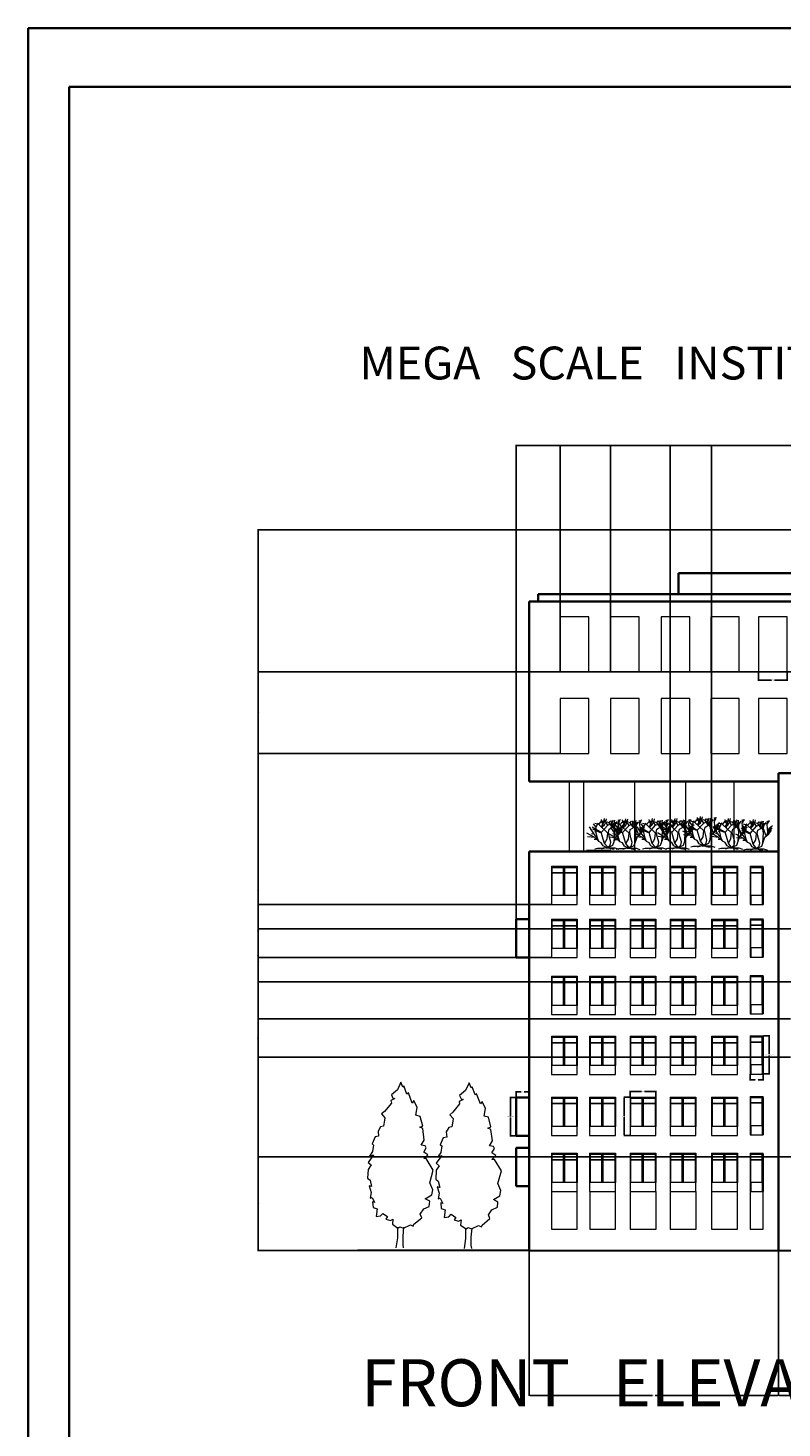
# Model space of a CAD drawing. Units: inches. Extents: x -279 to 364, y -385 to 335.
# Tile 5 of 9: x -279 to -60, y -72 to 335. Entities that reach past the tile are written whole.
import ezdxf

# ---------------------------------------------------------------- set-up
doc = ezdxf.new("R2010")
doc.units = ezdxf.units.IN
doc.header["$MEASUREMENT"] = 0
for name, color, linetype, lineweight in [('A-ANNO-DIMS', 2, 'Continuous', 18), ('A-ANNO-TEXT', 7, 'Continuous', 25), ('A-ANNO-TTLB', 7, 'Continuous', 35), ('A-GLAZ', 4, 'Continuous', 18), ('A-GLAZ-CURT', 4, 'Continuous', 18), ('A-ROOF', 7, 'Continuous', 35), ('A-WALL', 7, 'Continuous', 35), ('C-TOPO', 32, 'Continuous', 30), ('L-PLNT', 94, 'Continuous', 13)]:
    doc.layers.add(name, color=color, linetype=linetype, lineweight=lineweight)
doc.styles.get("Standard").update_dxf_attribs({"font": 'arial.ttf'})
doc.dimstyles.get("Standard").update_dxf_attribs({"dimtxt": 0.18, "dimasz": 0.18, "dimexe": 0.18, "dimexo": 0.0625, "dimgap": 0.09, "dimtad": 0, "dimtih": 1, "dimtoh": 1, "dimdec": 4, "dimzin": 0, "dimdsep": 46, "dimtxsty": 'Standard', "dimcen": 0.09, "dimadec": 0, "dimazin": 0, "dimtfac": 1, "dimtdec": 4, "dimtofl": 0, "dimtmove": 0, "dimatfit": 3, "dimfxl": 1, "dimtolj": 1, "dimtzin": 0, "dimarcsym": 0})

# ---------------------------------------------------------------- blocks, each defined once
blk = doc.blocks.new('*U2')
for p, q in [((-12.471, 19.775), (-12.898, 22.044)), ((-11.28, 19.619), (-12.104, 21.184)), ((-11.433, 18.289), (-10.457, 22.749)), ((-8.16, 17.76), (-10.56, 21.6)), ((-9.48, 19.775), (-8.992, 22.592)), ((-7.2, 19.68), (-6.24, 21.12)), ((-5.086, 17.741), (-5.513, 21.34)), ((-5.28, 19.2), (-3.84, 21.6)), ((-3.377, 18.602), (-2.888, 21.575)), ((-0.508, 21.888), (-0.081, 20.558)), ((-0.203, 19.149), (0.102, 21.34)), ((-0.02, 20.01), (0.896, 21.105)), ((0.041, 20.714), (1.384, 22.044)), ((0.102, 21.34), (0.835, 21.888)), ((-17.76, 8.64), (-23.663, 11.961)), ((-18.24, 11.04), (-21.755, 16.655)), ((-18.24, 11.04), (-20.16, 11.52)), ((-12.96, 12.48), (-19.68, 16.32)), ((-13.92, 12.48), (-19.2, 14.88)), ((-16.8, 16.32), (-18.72, 18.72)), ((-15.84, 8.16), (-18.24, 11.04)), ((-14.88, 18.24), (-17.76, 19.2)), ((-16.8, 12.48), (-17.76, 12.96)), ((-16.8, 16.32), (-15.36, 19.68)), ((-16.8, 12.48), (-16.8, 16.32)), ((-15.84, 8.16), (-16.8, 12.48)), ((-14.88, 18.24), (-12.96, 20.64)), ((-8.16, 12), (-14.88, 18.24)), ((-12.96, 12.48), (-13.92, 12.48)), ((-13.325, 16.724), (-11.433, 18.289)), ((-12.96, 12.48), (-8.16, 17.76)), ((-10.56, 4.32), (-12.96, 12.48)), ((-11.677, 19.071), (-12.471, 19.775)), ((-12.043, 15.628), (-11.921, 18.836)), ((-11.982, 16.802), (-10.579, 18.054)), ((-11.921, 18.836), (-10.64, 20.401)), ((-10.579, 18.054), (-9.846, 19.697)), ((-7.2, 19.68), (-8.64, 20.16)), ((-8.64, 7.68), (-8.16, 12)), ((-8.16, 17.76), (-5.28, 19.2)), ((-7.68, 12.48), (-7.2, 14.88)), ((-6.72, 8.64), (-7.68, 12.48)), ((-4.8, 16.32), (-7.2, 19.68)), ((-7.2, 14.88), (-3.84, 16.8)), ((-3.377, 15.315), (-5.086, 17.819)), ((-2.88, 12.96), (-4.32, 19.68)), ((-3.84, 16.8), (-0.96, 20.64)), ((-2.766, 16.802), (-3.377, 18.602)), ((-3.36, 5.28), (-2.88, 12.96)), ((-2.88, 15.84), (-2.4, 20.16)), ((-0.96, 10.56), (-2.88, 15.84)), ((-1.92, 9.6), (0.96, 12)), ((-0.48, 10.8), (0.346, 13.203)), ((0.346, 13.203), (-0.203, 19.149)), ((-0.142, 19.384), (0.59, 20.401)), ((0.346, 13.203), (1.323, 16.254)), ((0.96, 12), (1.44, 15.36)), ((0.96, 12), (2.88, 14.88)), ((1.323, 16.254), (3.642, 18.289)), ((1.44, 15.36), (2.88, 17.28)), ((1.92, 13.44), (2.4, 15.36)), ((2.4, 15.36), (3.36, 16.32)), ((-17.76, 8.64), (-23.128, 9.222)), ((-16.32, 7.2), (-18.24, 7.2)), ((-14.88, 5.76), (-17.76, 8.64)), ((-15.84, 0.48), (-17.76, 0)), ((-14.88, 5.76), (-15.84, 8.16)), ((-13.44, 0.48), (-15.84, 0.48)), ((-12.96, 4.8), (-14.88, 5.76)), ((-9.6, 0.96), (-13.44, 0.48)), ((-11.52, 2.4), (-12.96, 4.8)), ((-9.6, 0.96), (-12.96, 0)), ((-8.64, 0.96), (-11.52, 2.4)), ((-10.56, 4.32), (-8.64, 7.68)), ((-8.64, 1.92), (-10.56, 4.32)), ((-9.6, 0.96), (-7.68, 0.96)), ((-8.64, 0.96), (-4.32, 2.88)), ((-8.64, 0.96), (-6.24, 2.88)), ((-8.64, 0.96), (-8.64, 1.92)), ((-8.64, 0.96), (-2.88, 0.96)), ((-7.68, 0.96), (-6.24, 0.48)), ((-5.76, 5.28), (-6.72, 8.64)), ((-6.24, 2.88), (-5.76, 5.28)), ((-6.24, 0.48), (-3.36, 0)), ((-4.32, 2.88), (-1.92, 9.6)), ((-2.88, 0.96), (0, 0))]:
    blk.add_line(p, q)
blk = doc.blocks.new('*U3')
blk.add_lwpolyline([(-2.754, 191.699), (-6.78, 182.851), (-13.682, 176.953), (-11.956, 173.266), (-9.656, 172.529), (-14.257, 170.317), (-13.682, 167.368), (-21.733, 157.783), (-25.184, 154.834), (-21.158, 150.41), (-21.733, 147.461), (-22.884, 140.825), (-26.334, 140.087), (-29.21, 134.926), (-28.635, 129.028), (-32.661, 128.291), (-36.111, 120.18), (-34.386, 118.706), (-35.536, 111.333), (-38.987, 106.171), (-34.386, 107.646), (-40.712, 98.798), (-37.261, 95.849), (-40.712, 90.688), (-41.287, 80.366), (-38.412, 78.154), (-36.686, 70.781), (-39.562, 71.518), (-37.261, 64.145), (-38.412, 57.509), (-36.111, 58.247), (-33.236, 52.348), (-35.536, 53.086), (-34.961, 46.45), (-30.36, 44.975), (-31.51, 36.128), (-26.334, 36.865), (-23.459, 39.814), (-18.283, 36.128), (-20.008, 33.178), (-14.832, 31.704), (-11.956, 33.178), (-12.531, 27.28), (-6.205, 22.856), (-3.905, 24.331), (0.121, 22.856), (8.173, 26.543), (11.624, 25.068), (12.199, 27.28), (21.4, 34.653), (19.675, 39.077), (23.701, 44.975), (30.027, 47.924), (30.602, 53.823), (25.426, 56.772), (32.903, 61.196), (34.053, 67.094), (30.602, 75.205), (34.628, 89.951), (26.576, 103.222), (23.701, 103.222), (28.302, 107.646), (23.701, 110.595), (26.576, 115.756), (25.426, 117.968), (20.825, 118.706), (24.276, 124.604), (22.551, 137.876), (19.1, 139.35), (22.551, 140.825), (19.675, 151.884), (14.499, 153.359), (16.224, 162.207), (12.199, 170.317), (10.473, 167.368), (5.872, 179.165), (4.147, 177.69), (0.696, 187.275), (-0.454, 185.8)], close=True)
for points in [[(-6.813, 23.669), (-6.813, 11.669), (-8.627, 0)], [(0.387, 23.669), (-0.576, 13.271), (-0.576, 3.686), (0, 0)]]:
    blk.add_lwpolyline(points)
blk = doc.blocks.new('WIN-WING-NARROW')
for p, q in [((0, 11.12), (0, 0)), ((0, 11.12), (3.85, 11.12)), ((0.2, 2.62), (0.2, 10.81)), ((0.2, 10.81), (3.85, 10.81)), ((0.2, 9.34), (3.52, 9.34)), ((0.2, 9.24), (3.52, 9.24)), ((3.52, 9.34), (3.52, 10.81)), ((3.52, 2.62), (3.52, 9.24)), ((3.85, 9.24), (3.85, 11.12)), ((3.85, 10.81), (3.85, 9.34)), ((3.85, 9.24), (3.85, 2.62)), ((3.85, 2.62), (0, 2.62)), ((0, 0), (3.85, 0)), ((0.2, 2.62), (0.2, 0)), ((3.52, 2.62), (3.52, 0)), ((3.85, 2.62), (3.85, 0))]:
    blk.add_line(p, q)
blk = doc.blocks.new('WIN-TOWER-FRONT')
for p, q in [((8.3, 15.93), (0, 15.93)), ((0, 15.93), (0, 14.74)), ((0, 14.74), (0, 0)), ((8.3, 0), (8.3, 15.93)), ((0, 0), (8.3, 0))]:
    blk.add_line(p, q)
blk = doc.blocks.new('WING-RETURN-SHORT')
for p, q in [((3.76, 11.12), (0, 11.12)), ((0, 11.12), (0, 0)), ((0, 0), (3.76, 0))]:
    blk.add_line(p, q)
blk = doc.blocks.new('WIN-WING-TWIN')
for p, q in [((0, 11.12), (0, 0)), ((0, 11.12), (7.53, 11.12)), ((0.2, 2.62), (0.2, 10.81)), ((0.2, 10.81), (7.32, 10.81)), ((0.2, 9.34), (3.52, 9.34)), ((0.2, 9.24), (3.52, 9.24)), ((3.52, 9.34), (3.52, 10.81)), ((3.52, 2.62), (3.52, 9.24)), ((3.85, 10.81), (3.85, 9.34)), ((3.85, 9.34), (7.32, 9.34)), ((3.85, 9.24), (7.32, 9.24)), ((3.85, 9.24), (3.85, 2.62)), ((7.32, 10.81), (7.32, 2.62)), ((7.53, 11.12), (7.53, 2.62)), ((7.53, 2.62), (0, 2.62)), ((0, 0), (7.53, 0)), ((7.53, 0), (7.53, 2.62))]:
    blk.add_line(p, q)
blk = doc.blocks.new('*D30')
at = {"layer": 'A-ANNO-DIMS', "color": 0, "lineweight": -2, "transparency": 16777216}
for p, q in [((-104.61, 24.4), (-106.39, 24.4)), ((-106.21, 24.22), (-106.21, 19.02)), ((-106.21, 13.46), (-106.21, 18.66)), ((-104.61, 13.28), (-106.39, 13.28))]:
    blk.add_line(p, q, dxfattribs=at)
at = {"layer": 'A-ANNO-DIMS', "color": 0, "transparency": 16777216}
for points in [[(-106.24, 24.22), (-106.18, 24.22), (-106.21, 24.4)], [(-106.24, 13.46), (-106.18, 13.46), (-106.21, 13.28)]]:
    blk.add_solid(points, dxfattribs=at)
at = {"layer": 'Defpoints', "color": 0, "transparency": 16777216}
for p in [(-106.21, 24.4), (-104.55, 24.4), (-104.55, 13.28)]:
    blk.add_point(p, dxfattribs=at)
at = {"layer": 'A-ANNO-DIMS', "color": 0, "transparency": 16777216, "insert": (-106.21, 18.84), "char_height": 0.18, "attachment_point": 5}
blk.add_mtext('\\A1;PAIR 11 TYP.', dxfattribs=at)
blk = doc.blocks.new('*D31')
at = {"layer": 'A-ANNO-DIMS', "color": 0, "lineweight": -2, "transparency": 16777216}
for p, q in [((-104.55, 24.46), (-104.55, 26.25)), ((-104.37, 26.07), (-101.24, 26.07)), ((-97.2, 26.07), (-100.32, 26.07)), ((-97.02, 24.46), (-97.02, 26.25))]:
    blk.add_line(p, q, dxfattribs=at)
at = {"layer": 'A-ANNO-DIMS', "color": 0, "transparency": 16777216}
for points in [[(-104.37, 26.1), (-104.37, 26.04), (-104.55, 26.07)], [(-97.2, 26.1), (-97.2, 26.04), (-97.02, 26.07)]]:
    blk.add_solid(points, dxfattribs=at)
at = {"layer": 'Defpoints', "color": 0, "transparency": 16777216}
for p in [(-104.55, 24.4), (-97.02, 26.07), (-97.02, 24.4)]:
    blk.add_point(p, dxfattribs=at)
at = {"layer": 'A-ANNO-DIMS', "color": 0, "transparency": 16777216, "insert": (-100.78, 26.07), "char_height": 0.18, "attachment_point": 5}
blk.add_mtext('\\A1;8 TYP.', dxfattribs=at)
blk = doc.blocks.new('*D32')
at = {"layer": 'A-ANNO-DIMS', "color": 0, "lineweight": -2, "transparency": 16777216}
for p, q in [((-65.82, 42.24), (-64.03, 42.24)), ((-64.21, 42.06), (-64.21, 36.87)), ((-64.21, 31.31), (-64.21, 36.5)), ((-65.82, 31.13), (-64.03, 31.13))]:
    blk.add_line(p, q, dxfattribs=at)
at = {"layer": 'A-ANNO-DIMS', "color": 0, "transparency": 16777216}
for points in [[(-64.24, 42.06), (-64.18, 42.06), (-64.21, 42.24)], [(-64.24, 31.31), (-64.18, 31.31), (-64.21, 31.13)]]:
    blk.add_solid(points, dxfattribs=at)
at = {"layer": 'Defpoints', "color": 0, "transparency": 16777216}
for p in [(-65.88, 42.24), (-64.21, 42.24), (-65.88, 31.13)]:
    blk.add_point(p, dxfattribs=at)
at = {"layer": 'A-ANNO-DIMS', "color": 0, "transparency": 16777216, "insert": (-64.21, 36.68), "char_height": 0.18, "attachment_point": 5}
blk.add_mtext('\\A1;NARROW SASH 11 TYP.', dxfattribs=at)
blk = doc.blocks.new('*D33')
at = {"layer": 'A-ANNO-DIMS', "color": 0, "lineweight": -2, "transparency": 16777216}
for p, q in [((-69.73, 31.06), (-69.73, 29.28)), ((-69.55, 29.46), (-68.26, 29.46)), ((-66.06, 29.46), (-67.34, 29.46)), ((-65.88, 31.06), (-65.88, 29.28))]:
    blk.add_line(p, q, dxfattribs=at)
at = {"layer": 'A-ANNO-DIMS', "color": 0, "transparency": 16777216}
for points in [[(-69.55, 29.49), (-69.55, 29.43), (-69.73, 29.46)], [(-66.06, 29.49), (-66.06, 29.43), (-65.88, 29.46)]]:
    blk.add_solid(points, dxfattribs=at)
at = {"layer": 'Defpoints', "color": 0, "transparency": 16777216}
for p in [(-69.73, 31.13), (-65.88, 31.13), (-65.88, 29.46)]:
    blk.add_point(p, dxfattribs=at)
at = {"layer": 'A-ANNO-DIMS', "color": 0, "transparency": 16777216, "insert": (-67.8, 29.46), "char_height": 0.18, "attachment_point": 5}
blk.add_mtext('\\A1;4 TYP.', dxfattribs=at)
blk = doc.blocks.new('*D35')
at = {"layer": 'A-ANNO-DIMS', "color": 0, "lineweight": -2, "transparency": 16777216}
for p, q in [((-67.23, 147.75), (-67.23, 145.25)), ((-58.93, 147.75), (-58.93, 145.25)), ((-67.05, 145.43), (-63.54, 145.43)), ((-59.11, 145.43), (-62.62, 145.43))]:
    blk.add_line(p, q, dxfattribs=at)
at = {"layer": 'A-ANNO-DIMS', "color": 0, "transparency": 16777216}
for points in [[(-67.05, 145.46), (-67.05, 145.4), (-67.23, 145.43)], [(-59.11, 145.46), (-59.11, 145.4), (-58.93, 145.43)]]:
    blk.add_solid(points, dxfattribs=at)
at = {"layer": 'Defpoints', "color": 0, "transparency": 16777216}
for p in [(-67.23, 147.82), (-58.93, 147.82), (-58.93, 145.43)]:
    blk.add_point(p, dxfattribs=at)
at = {"layer": 'A-ANNO-DIMS', "color": 0, "transparency": 16777216, "insert": (-63.08, 145.43), "char_height": 0.18, "attachment_point": 5}
blk.add_mtext('\\A1;8 TYP.', dxfattribs=at)
blk = doc.blocks.new('*D64')
at = {"layer": 'A-ANNO-DIMS', "color": 0, "lineweight": -2, "transparency": 16777216}
for p, q in [((-137.62, 24.27), (-139.41, 24.27)), ((-139.23, 24.09), (-139.23, 18.9)), ((-139.23, 13.34), (-139.23, 18.53)), ((-137.62, 13.16), (-139.41, 13.16))]:
    blk.add_line(p, q, dxfattribs=at)
at = {"layer": 'A-ANNO-DIMS', "color": 0, "transparency": 16777216}
for points in [[(-139.26, 24.09), (-139.2, 24.09), (-139.23, 24.27)], [(-139.26, 13.34), (-139.2, 13.34), (-139.23, 13.16)]]:
    blk.add_solid(points, dxfattribs=at)
at = {"layer": 'Defpoints', "color": 0, "transparency": 16777216}
for p in [(-139.23, 24.27), (-137.56, 24.27), (-137.56, 13.16)]:
    blk.add_point(p, dxfattribs=at)
at = {"layer": 'A-ANNO-DIMS', "color": 0, "transparency": 16777216, "insert": (-139.23, 18.71), "char_height": 0.18, "attachment_point": 5}
blk.add_mtext('\\A1;RETURN 11 TYP.', dxfattribs=at)
blk = doc.blocks.new('*D65')
at = {"layer": 'A-ANNO-DIMS', "color": 0, "lineweight": -2, "transparency": 16777216}
for p, q in [((-137.56, 24.33), (-137.56, 26.12)), ((-137.38, 25.94), (-136.14, 25.94)), ((-133.98, 25.94), (-135.22, 25.94)), ((-133.8, 24.33), (-133.8, 26.12))]:
    blk.add_line(p, q, dxfattribs=at)
at = {"layer": 'A-ANNO-DIMS', "color": 0, "transparency": 16777216}
for points in [[(-137.38, 25.97), (-137.38, 25.91), (-137.56, 25.94)], [(-133.98, 25.97), (-133.98, 25.91), (-133.8, 25.94)]]:
    blk.add_solid(points, dxfattribs=at)
at = {"layer": 'Defpoints', "color": 0, "transparency": 16777216}
for p in [(-133.8, 25.94), (-137.56, 24.27), (-133.8, 24.27)]:
    blk.add_point(p, dxfattribs=at)
at = {"layer": 'A-ANNO-DIMS', "color": 0, "transparency": 16777216, "insert": (-135.68, 25.94), "char_height": 0.18, "attachment_point": 5}
blk.add_mtext('\\A1;4 TYP.', dxfattribs=at)
blk = doc.blocks.new('*D74')
at = {"layer": 'A-ANNO-DIMS', "color": 0, "lineweight": -2, "transparency": 16777216}
for p, q in [((-137.56, 76.08), (-137.56, 213.67)), ((-137.38, 213.49), (54.29, 213.49)), ((246.75, 213.49), (55.08, 213.49)), ((246.93, 76.27), (246.93, 213.67))]:
    blk.add_line(p, q, dxfattribs=at)
at = {"layer": 'A-ANNO-DIMS', "color": 0, "transparency": 16777216}
for points in [[(-137.38, 213.52), (-137.38, 213.46), (-137.56, 213.49)], [(246.75, 213.52), (246.75, 213.46), (246.93, 213.49)]]:
    blk.add_solid(points, dxfattribs=at)
at = {"layer": 'Defpoints', "color": 0, "transparency": 16777216}
for p in [(246.93, 213.49), (-137.56, 76.01), (246.93, 76.21)]:
    blk.add_point(p, dxfattribs=at)
at = {"layer": 'A-ANNO-DIMS', "color": 0, "transparency": 16777216, "insert": (54.68, 213.49), "char_height": 0.18, "attachment_point": 5}
blk.add_mtext('\\A1;384.5', dxfattribs=at)
blk = doc.blocks.new('*D75')
at = {"layer": 'A-ANNO-DIMS', "color": 0, "lineweight": -2, "transparency": 16777216}
for p, q in [((53.76, 188.99), (-212.62, 188.99)), ((-212.44, 188.81), (-212.44, 84.64)), ((-212.44, -19.9), (-212.44, 84.27)), ((-133.86, -20.08), (-212.62, -20.08))]:
    blk.add_line(p, q, dxfattribs=at)
at = {"layer": 'A-ANNO-DIMS', "color": 0, "transparency": 16777216}
for points in [[(-212.47, 188.81), (-212.41, 188.81), (-212.44, 188.99)], [(-212.47, -19.9), (-212.41, -19.9), (-212.44, -20.08)]]:
    blk.add_solid(points, dxfattribs=at)
at = {"layer": 'Defpoints', "color": 0, "transparency": 16777216}
for p in [(-212.44, 188.99), (53.82, 188.99), (-133.8, -20.08)]:
    blk.add_point(p, dxfattribs=at)
at = {"layer": 'A-ANNO-DIMS', "color": 0, "transparency": 16777216, "insert": (-212.44, 84.45), "char_height": 0.18, "attachment_point": 5}
blk.add_mtext('\\A1;209.07', dxfattribs=at)
blk = doc.blocks.new('*D76')
at = {"layer": 'A-ANNO-DIMS', "color": 0, "lineweight": -2, "transparency": 16777216}
for p, q in [((17.12, 147.82), (-212.62, 147.82)), ((-212.44, 147.64), (-212.44, 64.05)), ((-212.44, -19.9), (-212.44, 63.68)), ((17.4, -20.08), (-212.62, -20.08))]:
    blk.add_line(p, q, dxfattribs=at)
at = {"layer": 'A-ANNO-DIMS', "color": 0, "transparency": 16777216}
for points in [[(-212.47, 147.64), (-212.41, 147.64), (-212.44, 147.82)], [(-212.47, -19.9), (-212.41, -19.9), (-212.44, -20.08)]]:
    blk.add_solid(points, dxfattribs=at)
at = {"layer": 'Defpoints', "color": 0, "transparency": 16777216}
for p in [(-212.44, 147.82), (17.19, 147.82), (17.46, -20.08)]:
    blk.add_point(p, dxfattribs=at)
at = {"layer": 'A-ANNO-DIMS', "color": 0, "transparency": 16777216, "insert": (-212.44, 63.87), "char_height": 0.18, "attachment_point": 5}
blk.add_mtext('\\A1;167.9', dxfattribs=at)
blk = doc.blocks.new('*D77')
at = {"layer": 'A-ANNO-DIMS', "color": 0, "lineweight": -2, "transparency": 16777216}
for p, q in [((-133.8, -20.14), (-133.8, -62.3)), ((-61.49, -20.14), (-61.49, -62.3)), ((-133.62, -62.12), (-98.02, -62.12)), ((-61.67, -62.12), (-97.27, -62.12))]:
    blk.add_line(p, q, dxfattribs=at)
at = {"layer": 'A-ANNO-DIMS', "color": 0, "transparency": 16777216}
for points in [[(-133.62, -62.09), (-133.62, -62.15), (-133.8, -62.12)], [(-61.67, -62.09), (-61.67, -62.15), (-61.49, -62.12)]]:
    blk.add_solid(points, dxfattribs=at)
at = {"layer": 'Defpoints', "color": 0, "transparency": 16777216}
for p in [(-133.8, -20.08), (-61.49, -20.08), (-61.49, -62.12)]:
    blk.add_point(p, dxfattribs=at)
at = {"layer": 'A-ANNO-DIMS', "color": 0, "transparency": 16777216, "insert": (-97.64, -62.12), "char_height": 0.18, "attachment_point": 5}
blk.add_mtext('\\A1;72.31', dxfattribs=at)
blk = doc.blocks.new('*D78')
at = {"layer": 'A-ANNO-DIMS', "color": 0, "lineweight": -2, "transparency": 16777216}
for p, q in [((-61.49, -20.14), (-61.49, -62.3)), ((13.58, -20.14), (13.58, -62.3)), ((-61.31, -62.12), (-24.34, -62.12)), ((13.4, -62.12), (-23.56, -62.12))]:
    blk.add_line(p, q, dxfattribs=at)
at = {"layer": 'A-ANNO-DIMS', "color": 0, "transparency": 16777216}
for points in [[(-61.31, -62.09), (-61.31, -62.15), (-61.49, -62.12)], [(13.4, -62.09), (13.4, -62.15), (13.58, -62.12)]]:
    blk.add_solid(points, dxfattribs=at)
at = {"layer": 'Defpoints', "color": 0, "transparency": 16777216}
for p in [(-61.49, -20.08), (13.58, -20.08), (13.58, -62.12)]:
    blk.add_point(p, dxfattribs=at)
at = {"layer": 'A-ANNO-DIMS', "color": 0, "transparency": 16777216, "insert": (-23.95, -62.12), "char_height": 0.18, "attachment_point": 5}
blk.add_mtext('\\A1;75.07', dxfattribs=at)
blk = doc.blocks.new('*D85')
at = {"layer": 'A-ANNO-DIMS', "color": 0, "lineweight": -2, "transparency": 16777216}
for p, q in [((-124.8, 147.88), (-124.8, 213.67)), ((-124.62, 213.49), (-117.91, 213.49)), ((-110.43, 213.49), (-117.14, 213.49)), ((-110.25, 147.88), (-110.25, 213.67))]:
    blk.add_line(p, q, dxfattribs=at)
at = {"layer": 'A-ANNO-DIMS', "color": 0, "transparency": 16777216}
for points in [[(-124.62, 213.52), (-124.62, 213.46), (-124.8, 213.49)], [(-110.43, 213.52), (-110.43, 213.46), (-110.25, 213.49)]]:
    blk.add_solid(points, dxfattribs=at)
at = {"layer": 'Defpoints', "color": 0, "transparency": 16777216}
for p in [(-110.25, 213.49), (-124.8, 147.82), (-110.25, 147.82)]:
    blk.add_point(p, dxfattribs=at)
at = {"layer": 'A-ANNO-DIMS', "color": 0, "transparency": 16777216, "insert": (-117.52, 213.49), "char_height": 0.18, "attachment_point": 5}
blk.add_mtext('\\A1;14.55', dxfattribs=at)
blk = doc.blocks.new('*D86')
at = {"layer": 'A-ANNO-DIMS', "color": 0, "lineweight": -2, "transparency": 16777216}
for p, q in [((-124.86, 147.82), (-212.62, 147.82)), ((-212.44, 147.64), (-212.44, 136.17)), ((-212.44, 124.35), (-212.44, 135.81)), ((-124.86, 124.17), (-212.62, 124.17))]:
    blk.add_line(p, q, dxfattribs=at)
at = {"layer": 'A-ANNO-DIMS', "color": 0, "transparency": 16777216}
for points in [[(-212.47, 147.64), (-212.41, 147.64), (-212.44, 147.82)], [(-212.47, 124.35), (-212.41, 124.35), (-212.44, 124.17)]]:
    blk.add_solid(points, dxfattribs=at)
at = {"layer": 'Defpoints', "color": 0, "transparency": 16777216}
for p in [(-212.44, 147.82), (-124.8, 147.82), (-124.8, 124.17)]:
    blk.add_point(p, dxfattribs=at)
at = {"layer": 'A-ANNO-DIMS', "color": 0, "transparency": 16777216, "insert": (-212.44, 135.99), "char_height": 0.18, "attachment_point": 5}
blk.add_mtext('\\A1;23.646', dxfattribs=at)
blk = doc.blocks.new('*D87')
at = {"layer": 'A-ANNO-DIMS', "color": 0, "lineweight": -2, "transparency": 16777216}
for p, q in [((-92.95, 80.34), (-92.95, 213.67)), ((-92.77, 213.49), (-87.37, 213.49)), ((-81.05, 213.49), (-86.46, 213.49)), ((-80.87, 80.34), (-80.87, 213.67))]:
    blk.add_line(p, q, dxfattribs=at)
at = {"layer": 'A-ANNO-DIMS', "color": 0, "transparency": 16777216}
for points in [[(-92.77, 213.52), (-92.77, 213.46), (-92.95, 213.49)], [(-81.05, 213.52), (-81.05, 213.46), (-80.87, 213.49)]]:
    blk.add_solid(points, dxfattribs=at)
at = {"layer": 'Defpoints', "color": 0, "transparency": 16777216}
for p in [(-80.87, 213.49), (-92.95, 80.27), (-80.87, 80.27)]:
    blk.add_point(p, dxfattribs=at)
at = {"layer": 'A-ANNO-DIMS', "color": 0, "transparency": 16777216, "insert": (-86.91, 213.49), "char_height": 0.18, "attachment_point": 5}
blk.add_mtext('\\A1;12.082', dxfattribs=at)
blk = doc.blocks.new('*D88')
at = {"layer": 'A-ANNO-DIMS', "color": 0, "lineweight": -2, "transparency": 16777216}
for p, q in [((-127.43, 80.27), (-212.62, 80.27)), ((-212.44, 80.09), (-212.44, 72.77)), ((-212.44, 65.08), (-212.44, 72.4)), ((-127.43, 64.9), (-212.62, 64.9))]:
    blk.add_line(p, q, dxfattribs=at)
at = {"layer": 'A-ANNO-DIMS', "color": 0, "transparency": 16777216}
for points in [[(-212.47, 80.09), (-212.41, 80.09), (-212.44, 80.27)], [(-212.47, 65.08), (-212.41, 65.08), (-212.44, 64.9)]]:
    blk.add_solid(points, dxfattribs=at)
at = {"layer": 'Defpoints', "color": 0, "transparency": 16777216}
for p in [(-127.37, 80.27), (-212.44, 64.9), (-127.37, 64.9)]:
    blk.add_point(p, dxfattribs=at)
at = {"layer": 'A-ANNO-DIMS', "color": 0, "transparency": 16777216, "insert": (-212.44, 72.59), "char_height": 0.18, "attachment_point": 5}
blk.add_mtext('\\A1;15.377', dxfattribs=at)
blk = doc.blocks.new('*D90')
at = {"layer": 'A-ANNO-DIMS', "color": 0, "lineweight": -2, "transparency": 16777216}
for p, q in [((-58.02, 47.17), (-212.62, 47.17)), ((-212.44, 46.99), (-212.44, 41.78)), ((-212.44, 36.2), (-212.44, 41.41)), ((-58.02, 36.02), (-212.62, 36.02))]:
    blk.add_line(p, q, dxfattribs=at)
at = {"layer": 'A-ANNO-DIMS', "color": 0, "transparency": 16777216}
for points in [[(-212.47, 46.99), (-212.41, 46.99), (-212.44, 47.17)], [(-212.47, 36.2), (-212.41, 36.2), (-212.44, 36.02)]]:
    blk.add_solid(points, dxfattribs=at)
at = {"layer": 'Defpoints', "color": 0, "transparency": 16777216}
for p in [(-57.96, 47.17), (-212.44, 36.02), (-57.96, 36.02)]:
    blk.add_point(p, dxfattribs=at)
at = {"layer": 'A-ANNO-DIMS', "color": 0, "transparency": 16777216, "insert": (-212.44, 41.59), "char_height": 0.18, "attachment_point": 5}
blk.add_mtext('\\A1;11.149', dxfattribs=at)
blk = doc.blocks.new('*D91')
at = {"layer": 'A-ANNO-DIMS', "color": 0, "lineweight": -2, "transparency": 16777216}
for p, q in [((-48.59, 73.23), (-212.62, 73.23)), ((-212.44, 73.05), (-212.44, 65.74)), ((-212.44, 58.07), (-212.44, 65.38)), ((-48.59, 57.89), (-212.62, 57.89))]:
    blk.add_line(p, q, dxfattribs=at)
at = {"layer": 'A-ANNO-DIMS', "color": 0, "transparency": 16777216}
for points in [[(-212.47, 73.05), (-212.41, 73.05), (-212.44, 73.23)], [(-212.47, 58.07), (-212.41, 58.07), (-212.44, 57.89)]]:
    blk.add_solid(points, dxfattribs=at)
at = {"layer": 'Defpoints', "color": 0, "transparency": 16777216}
for p in [(-212.44, 73.23), (-48.53, 73.23), (-48.53, 57.89)]:
    blk.add_point(p, dxfattribs=at)
at = {"layer": 'A-ANNO-DIMS', "color": 0, "transparency": 16777216, "insert": (-212.44, 65.56), "char_height": 0.18, "attachment_point": 5}
blk.add_mtext('\\A1;15.345', dxfattribs=at)
blk = doc.blocks.new('*D94')
at = {"layer": 'A-ANNO-DIMS', "color": 0, "lineweight": -2, "transparency": 16777216}
for p, q in [((-21.25, 7.08), (-212.62, 7.08)), ((-212.44, 6.9), (-212.44, -6.32)), ((-212.44, -19.9), (-212.44, -6.68)), ((-21.25, -20.08), (-212.62, -20.08))]:
    blk.add_line(p, q, dxfattribs=at)
at = {"layer": 'A-ANNO-DIMS', "color": 0, "transparency": 16777216}
for points in [[(-212.47, 6.9), (-212.41, 6.9), (-212.44, 7.08)], [(-212.47, -19.9), (-212.41, -19.9), (-212.44, -20.08)]]:
    blk.add_solid(points, dxfattribs=at)
at = {"layer": 'Defpoints', "color": 0, "transparency": 16777216}
for p in [(-212.44, 7.08), (-21.19, 7.08), (-21.19, -20.08)]:
    blk.add_point(p, dxfattribs=at)
at = {"layer": 'A-ANNO-DIMS', "color": 0, "transparency": 16777216, "insert": (-212.44, -6.5), "char_height": 0.18, "attachment_point": 5}
blk.add_mtext('\\A1;27.16', dxfattribs=at)

msp = doc.modelspace()

# ---------------------------------------------------------------- linework, layer by layer
at = {"layer": 'A-ANNO-TTLB'}
for points in [[(-279.2289, 334.6468), (364.0508, 334.6468), (364.0508, -385.2219), (-279.2289, -385.2219)], [(-267.2403, 317.5778), (348.1051, 317.5778), (348.1051, -370.8321), (-267.2403, -370.8321)]]:
    msp.add_lwpolyline(points, close=True, dxfattribs=at)
at = {"layer": 'A-GLAZ'}
for p, q in [((-69.7256, 8.127), (-69.7256, -2.9883)), ((-69.7256, 8.127), (-65.8798, 8.127)), ((-65.8798, 6.254), (-65.8798, 8.127)), ((-69.5216, -0.373), (-69.5216, 7.8215)), ((-69.5216, 7.8215), (-65.8798, 7.8215)), ((-69.5216, 6.356), (-66.2083, 6.356)), ((-69.5216, 6.254), (-66.2083, 6.254)), ((-66.2083, 6.356), (-66.2083, 7.8215)), ((-66.2083, -0.373), (-66.2083, 6.254)), ((-65.8798, 7.8215), (-65.8798, 6.356)), ((-65.8798, 6.254), (-65.8798, -0.373)), ((-127.372, -2.982), (-127.372, -13.8647)), ((-119.8438, -13.8647), (-119.8438, -2.982)), ((-116.2608, -2.982), (-116.2608, -13.8647)), ((-108.7326, -13.8647), (-108.7326, -2.982)), ((-104.5416, -2.982), (-104.5416, -13.8647)), ((-97.0133, -13.8647), (-97.0133, -2.982)), ((-92.9153, -2.982), (-92.9153, -13.8647)), ((-85.3871, -13.8647), (-85.3871, -2.982)), ((-80.8963, -2.982), (-80.8963, -13.8647)), ((-73.3681, -13.8647), (-73.3681, -2.982)), ((-65.8798, -0.373), (-69.7256, -0.373)), ((-69.7256, -2.9883), (-65.8798, -2.9883)), ((-69.7256, -2.9883), (-69.7256, -13.8647)), ((-69.5216, -0.373), (-69.5216, -2.9883)), ((-66.2083, -0.373), (-66.2083, -2.9883)), ((-65.8798, -0.373), (-65.8798, -2.9883)), ((-65.8798, -13.8647), (-65.8798, -2.9883)), ((-127.372, -13.8647), (-119.8438, -13.8647)), ((-116.2608, -13.8647), (-108.7326, -13.8647)), ((-104.5416, -13.8647), (-97.0133, -13.8647)), ((-92.9153, -13.8647), (-85.3871, -13.8647)), ((-80.8963, -13.8647), (-73.3681, -13.8647)), ((-69.7256, -13.8647), (-65.8798, -13.8647)), ((-65.8798, -13.8647), (-65.8798, -13.8647))]:
    msp.add_line(p, q, dxfattribs=at)
at = {"layer": 'A-GLAZ-CURT'}
for p, q in [((-122.191, 115.9949), (-122.191, 95.7114)), ((-117.9144, 95.7114), (-117.9144, 115.9949)), ((-103.2605, 115.9949), (-103.2605, 95.7114)), ((-88.41, 115.9949), (-88.41, 95.7114)), ((-74.4384, 115.9949), (-74.4384, 95.7114))]:
    msp.add_line(p, q, dxfattribs=at)
at = {"layer": 'A-ROOF'}
for p, q in [((-90.5255, 170.3156), (-90.5255, 176.4444)), ((-90.5255, 176.4444), (-32.6709, 176.4444)), ((-131.1712, 168.1874), (-131.1712, 170.3156)), ((-131.1712, 170.3156), (-25.7643, 170.3156))]:
    msp.add_line(p, q, dxfattribs=at)
at = {"layer": 'A-WALL'}
for p, q in [((-133.7987, 115.9949), (-133.7987, 168.1874)), ((-133.7987, 168.1874), (-21.4109, 168.1874)), ((-61.4888, -2.9883), (-61.4888, 118.4445)), ((-61.4888, 118.4445), (13.5848, 118.4445)), ((-61.4888, 115.9949), (-133.7987, 115.9949)), ((-133.7987, 95.7114), (-133.7987, -2.6746)), ((-133.7987, 95.7114), (-68.6158, 95.7114)), ((-110.0787, 95.9049), (-117.2057, 95.9049)), ((-68.6158, 95.7114), (-61.4888, 95.7114)), ((-133.7987, -2.6746), (-133.7987, -20.0818)), ((-61.4888, -2.9883), (-61.4888, -20.0818))]:
    msp.add_line(p, q, dxfattribs=at)
at = {"layer": 'C-TOPO'}
for q in [(-183.5719, -20.0818), (198.4631, -20.0818)]:
    msp.add_line((-133.7987, -20.0818), q, dxfattribs=at)

# ---------------------------------------------------------------- block references
at = {"layer": 'A-GLAZ'}
for name, p in [('WIN-TOWER-FRONT', (-124.796, 147.815)), ('WIN-TOWER-FRONT', (-110.2469, 147.815)), ('WIN-TOWER-FRONT', (-95.487, 147.815)), ('WIN-TOWER-FRONT', (-81.1487, 147.815)), ('WIN-TOWER-FRONT', (-67.2322, 147.815)), ('WIN-TOWER-FRONT', (-124.796, 124.1691)), ('WIN-TOWER-FRONT', (-110.2469, 124.1691)), ('WIN-TOWER-FRONT', (-95.487, 124.1691)), ('WIN-TOWER-FRONT', (-81.1487, 124.1691)), ('WIN-TOWER-FRONT', (-67.2322, 124.1691)), ('WIN-WING-TWIN', (-127.372, 80.274)), ('WIN-WING-TWIN', (-116.2629, 80.274)), ('WIN-WING-TWIN', (-104.5466, 80.274)), ('WIN-WING-TWIN', (-92.9524, 80.274)), ('WIN-WING-TWIN', (-80.8701, 80.274)), ('WIN-WING-NARROW', (-69.726, 80.274)), ('WIN-WING-TWIN', (-127.372, 64.8975)), ('WIN-WING-TWIN', (-116.2629, 64.8975)), ('WIN-WING-TWIN', (-104.5466, 64.8975)), ('WIN-WING-TWIN', (-92.9524, 64.8975)), ('WIN-WING-TWIN', (-80.8701, 64.8975)), ('WIN-WING-NARROW', (-69.726, 65.072)), ('WIN-WING-TWIN', (-127.372, 48.4298)), ('WIN-WING-TWIN', (-116.2629, 48.4298)), ('WIN-WING-TWIN', (-104.5466, 48.4298)), ('WIN-WING-TWIN', (-92.9524, 48.4298)), ('WIN-WING-TWIN', (-80.8701, 48.4298)), ('WIN-WING-NARROW', (-69.726, 48.6135)), ('WIN-WING-TWIN', (-127.372, 30.9743)), ('WIN-WING-TWIN', (-116.2629, 30.9743)), ('WIN-WING-TWIN', (-104.5466, 30.9743)), ('WIN-WING-TWIN', (-92.9524, 30.9743)), ('WIN-WING-TWIN', (-80.8701, 30.9743)), ('WIN-WING-NARROW', (-69.726, 31.1253)), ('WIN-WING-TWIN', (-127.372, 13.2834)), ('WIN-WING-TWIN', (-116.2629, 13.2834)), ('WIN-WING-TWIN', (-104.5466, 13.2834)), ('WIN-WING-TWIN', (-92.9524, 13.2834)), ('WIN-WING-TWIN', (-80.8701, 13.2834)), ('WIN-WING-NARROW', (-69.726, 13.4813)), ('WIN-WING-TWIN', (-127.372, -2.982)), ('WIN-WING-TWIN', (-116.2629, -2.982)), ('WIN-WING-TWIN', (-104.5466, -2.982)), ('WIN-WING-TWIN', (-92.9524, -2.982)), ('WIN-WING-TWIN', (-80.8701, -2.982))]:
    msp.add_blockref(name, p, dxfattribs=at)
at = {"layer": 'A-WALL'}
for p in [(-137.559, 64.897), (-137.559, 13.1559), (-137.559, -1.4495)]:
    msp.add_blockref('WING-RETURN-SHORT', p, dxfattribs=at)
at = {"layer": 'L-PLNT'}
for name, p, xscale, yscale, zscale in [('*U2', (-79.9798, 96.9652), 0.390298493085325, 0.390298493085325, 0.390298493085325), ('*U2', (-107.8397, 96.3663), 0.390298493085325, 0.390298493085325, 0.390298493085325), ('*U2', (-101.6581, 96.2861), 0.390298493085325, 0.390298493085325, 0.390298493085325), ('*U2', (-93.9771, 96.3663), 0.390298493085325, 0.390298493085325, 0.390298493085325), ('*U2', (-87.3822, 96.4031), 0.390298493085325, 0.390298493085325, 0.390298493085325), ('*U2', (-71.9045, 96.4031), 0.390298493085325, 0.390298493085325, 0.390298493085325), ('*U2', (-64.6618, 96.0904), 0.390298493085325, 0.390298493085325, 0.390298493085325), ('*U3', (-170.3426, -19.3016), 0.2508480261805224, 0.2508480261805224, 0.2508480261805224), ('*U3', (-150.5532, -19.5341), 0.2508480261805224, 0.2508480261805224, 0.2508480261805224)]:
    msp.add_blockref(name, p, dxfattribs=dict(at, xscale=xscale, yscale=yscale, zscale=zscale))

# ---------------------------------------------------------------- texts
at = {"layer": 'A-ANNO-TEXT'}
for s, height, p in [('MEGA   SCALE   INSTITUTIONAL   CAMPUS   COMPREHENSIVE   ELEVATION ', 9.539438, (-183.0703, 232.6637)), ('FRONT   ELEVATION   MAIN   ACADEMIC   COMPLEX', 13.648689, (-182.5362, -65.301))]:
    msp.add_text(s, height=height, dxfattribs=at).set_placement(p)

# ---------------------------------------------------------------- dimensions: what is measured, and where the dimension line sits
at = {"layer": 'A-ANNO-DIMS'}
for base, p1, p2, override, picture, middle in [((246.9255, 213.4896), (-137.5587, 76.0128), (246.9255, 76.2063), {"dimdec": 1, "dimlfac": 1, "dimrnd": 0, "dimzin": 0, "dimdsep": 46, "dimlunit": 2}, '*D74', (54.6834, 213.4896)), ((-110.2474, 213.4896), (-124.7965, 147.8151), (-110.2474, 147.8151), {"dimdec": 2, "dimlfac": 1, "dimrnd": 0, "dimzin": 0, "dimdsep": 46, "dimlunit": 2}, '*D85', (-117.5219, 213.4896)), ((-80.8701, 213.4896), (-92.9524, 80.274), (-80.8701, 80.274), {"dimdec": 3, "dimlfac": 1, "dimrnd": 0, "dimzin": 0, "dimdsep": 46, "dimlunit": 2}, '*D87', (-86.9113, 213.4896)), ((-61.4888, -62.1247), (-133.7987, -20.0818), (-61.4888, -20.0818), {"dimdec": 2, "dimlfac": 1, "dimrnd": 0, "dimzin": 0, "dimdsep": 46, "dimlunit": 2}, '*D77', (-97.6437, -62.1247)), ((13.5848, -62.1247), (-61.4888, -20.0818), (13.5848, -20.0818), {"dimdec": 2, "dimlfac": 1, "dimrnd": 0, "dimzin": 0, "dimdsep": 46, "dimlunit": 2}, '*D78', (-23.952, -62.1247))]:
    dim = msp.add_linear_dim(base=base, p1=p1, p2=p2, dimstyle='Standard', override=override, dxfattribs=at)
    dim.commit()
    dim.dimension.update_dxf_attribs({"geometry": picture, "text_midpoint": middle})
for base, p1, p2, override, picture, middle in [((-212.4386, 188.9896), (-133.7987, -20.0818), (53.8218, 188.9896), {"dimdec": 2, "dimlfac": 1, "dimrnd": 0, "dimzin": 0, "dimdsep": 46, "dimlunit": 2}, '*D75', (-212.4386, 84.4539)), ((-212.4386, 147.8151), (-124.7965, 124.1692), (-124.7965, 147.8151), {"dimdec": 3, "dimlfac": 1, "dimrnd": 0, "dimzin": 0, "dimdsep": 46, "dimlunit": 2}, '*D86', (-212.4386, 135.9922)), ((-212.4386, 147.8151), (17.4585, -20.0818), (17.1869, 147.8151), {"dimdec": 1, "dimlfac": 1, "dimrnd": 0, "dimzin": 0, "dimdsep": 46, "dimlunit": 2}, '*D76', (-212.4386, 63.8666)), ((-212.43857, 64.89748), (-127.37199, 80.27403), (-127.37199, 64.89748), {"dimdec": 3, "dimlfac": 1, "dimrnd": 0, "dimzin": 0, "dimdsep": 46, "dimlunit": 2}, '*D88', (-212.43857, 72.58575)), ((-212.4386, 73.2332), (-48.5304, 57.8883), (-48.5304, 73.2332), {"dimdec": 3, "dimlfac": 1, "dimrnd": 0, "dimzin": 0, "dimdsep": 46, "dimlunit": 2}, '*D91', (-212.4386, 65.5608)), ((-212.4386, 36.0194), (-57.9596, 47.1683), (-57.9596, 36.0194), {"dimdec": 3, "dimlfac": 1, "dimrnd": 0, "dimzin": 0, "dimdsep": 46, "dimlunit": 2}, '*D90', (-212.4386, 41.5939)), ((-212.4386, 7.0763), (-21.1877, -20.0818), (-21.1877, 7.0763), {"dimdec": 2, "dimlfac": 1, "dimrnd": 0, "dimzin": 0, "dimdsep": 46, "dimlunit": 2}, '*D94', (-212.4386, -6.5028))]:
    dim = msp.add_linear_dim(base=base, p1=p1, p2=p2, angle=90, dimstyle='Standard', override=override, dxfattribs=at)
    dim.commit()
    dim.dimension.update_dxf_attribs({"geometry": picture, "text_midpoint": middle})
for base, p1, p2, picture, middle in [((-58.9294, 145.4259), (-67.2327, 147.8151), (-58.9294, 147.8151), '*D35', (-63.081, 145.4259)), ((-65.8798, 29.4581), (-69.7256, 31.1254), (-65.8798, 31.1254), '*D33', (-67.8027, 29.4581)), ((-133.7987, 25.9391), (-137.5587, 24.2718), (-133.7987, 24.2718), '*D65', (-135.6787, 25.9391)), ((-97.0184, 26.0661), (-104.5466, 24.3988), (-97.0184, 24.3988), '*D31', (-100.7825, 26.0661))]:
    dim = msp.add_linear_dim(base=base, p1=p1, p2=p2, text='<> TYP.', dimstyle='Standard', override={"dimdec": 0, "dimlfac": 1, "dimrnd": 0, "dimzin": 0, "dimdsep": 46, "dimlunit": 2}, dxfattribs=at)
    dim.commit()
    dim.dimension.update_dxf_attribs({"geometry": picture, "text_midpoint": middle})
for base, p1, p2, text, picture, middle in [((-64.2125, 42.2407), (-65.8798, 31.1254), (-65.8798, 42.2407), 'NARROW SASH <> TYP.', '*D32', (-64.2125, 36.683)), ((-106.2139, 24.3988), (-104.5466, 13.2834), (-104.5466, 24.3988), 'PAIR <> TYP.', '*D30', (-106.2139, 18.8411)), ((-139.226, 24.2718), (-137.5587, 13.1564), (-137.5587, 24.2718), 'RETURN <> TYP.', '*D64', (-139.226, 18.7141))]:
    dim = msp.add_linear_dim(base=base, p1=p1, p2=p2, angle=90, text=text, dimstyle='Standard', override={"dimdec": 0, "dimlfac": 1, "dimrnd": 0, "dimzin": 0, "dimdsep": 46, "dimlunit": 2}, dxfattribs=at)
    dim.commit()
    dim.dimension.update_dxf_attribs({"geometry": picture, "text_midpoint": middle})

doc.saveas('drawing.dxf')
